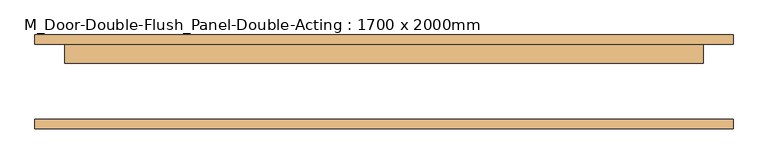
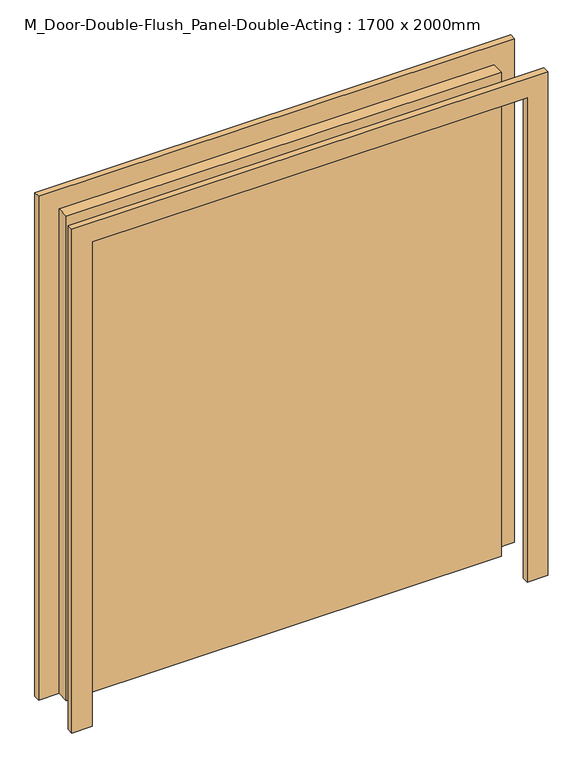
"""IFC4 building model written with IfcOpenShell, lengths in millimetres: door geometry, M_Door-Double-Flush_Panel-Double-Acting : 1700 x 2000mm."""

from ifc_helpers import new_model, si_unit, frame, origin, origin_with_axes, place, context, project, spatial, polyline, outline, extrude, source, transform, mapped, element, save


def m_door_double_flush_panel_double_acting_1700_x_2000mm_0a6d9c7f(model_context):
    return source(origin(), model_context, "Body", "SweptSolid", [
        extrude(outline(polyline([(2080.0, -930.0), (0.0, -930.0), (0.0, -850.0), (2000.0, -850.0), (2000.0, 850.0), (0.0, 850.0), (0.0, 930.0), (2080.0, 930.0), (2080.0, -930.0)])), frame((0.0, 100.0, 0.0), z_axis=(0.0, 1.0, 0.0), x_axis=(0.0, 0.0, 1.0)), (0.0, 0.0, 1.0), 25.0),
        extrude(outline(polyline([(2000.0, -850.0), (2000.0, 850.0), (0.0, 850.0), (0.0, 930.0), (2080.0, 930.0), (2080.0, -930.0), (0.0, -930.0), (0.0, -850.0), (2000.0, -850.0)])), frame((0.0, -125.0, 0.0), z_axis=(0.0, 1.0, 0.0), x_axis=(0.0, 0.0, 1.0)), (0.0, 0.0, 1.0), 25.0),
        extrude(outline(polyline([(-850.0, 100.0), (850.0, 100.0), (850.0, 50.0), (-850.0, 50.0), (-850.0, 100.0)])), origin_with_axes(), (0.0, 0.0, 1.0), 2000.0),
    ])


if __name__ == "__main__":
    model = new_model("IFC4")
    model_context = context("Model", 3, world=origin())
    ifc_project = project(units=[si_unit("LENGTHUNIT", "METRE", prefix="MILLI")], contexts=[model_context])
    site = spatial("IfcSite", under=ifc_project)
    building = spatial("IfcBuilding", under=site)
    placement = place(None, origin())
    m_door_double_flush_panel_double_acting_1700_x_2000mm_shape = m_door_double_flush_panel_double_acting_1700_x_2000mm_0a6d9c7f(model_context)
    element("IfcDoor", 1, ObjectType="M_Door-Double-Flush_Panel-Double-Acting : 1700 x 2000mm", at=placement, inside=building, context=model_context, shape_type="MappedRepresentation", body=[
        mapped(m_door_double_flush_panel_double_acting_1700_x_2000mm_shape, transform((0.0, 0.0, 0.0), x_axis=(1.0, 0.0, 0.0), y_axis=(0.0, 1.0, 0.0), z_axis=(0.0, 0.0, 1.0))),
    ])
    save(model, "model.ifc")

# Revit data of these elements
# Type "M_Door-Double-Flush_Panel-Double-Acting : 1700 x 2000mm"
#   Type Mark = "23"
#   Construction Type Id = "DOOR"
#   Assembly Code = "C1020"
#   Analytic Construction = "Wooden"
#   W = 2' - 9.46457"
#   Thickness = 0' - 1.9685"
#   Thermal Resistance (R) = 0.455703 (m²·K)/W
#   Swing Angle [instance default] = 90.00°
#   Heat Transfer Coefficient (U) = 2.19465 W/(m²·K)
#   Height = 6' - 6.74016"
#   Trim Projection Ext. = 0' - 0.98425"
#   Trim Projection Int. = 0' - 0.98425"
#   Trim Width Ext. = 0' - 3.14961"
#   Trim Width Int. = 0' - 3.14961"
#   Width = 5' - 6.92913"
#   Define Thermal Properties by = 1
#   Panel Material = Wood - Birch - Solid Stained Light Low Gloss
#   Trim Material = Paint - Sienna
#   Visual Light Transmittance = 0
#   Solar Heat Gain Coefficient = 0
#   Function = (empty or 0)
#   Wall Closure = (empty or 0)
# Element 1 (IfcDoor, "M_Door-Double-Flush_Panel-Double-Acting : 1700 x 2000mm")
#   Materials on its faces: "Paint - Sienna", "Wood - Birch - Solid Stained Light Low Gloss"
# Materials
#   "Wood - Birch - Solid Stained Light Low Gloss": class "Wood", colour RGB 210 159 95, transparency 0, Cost = 0
#   "Paint - Sienna": colour RGB 118 70 51, transparency 0, Cost = 0
